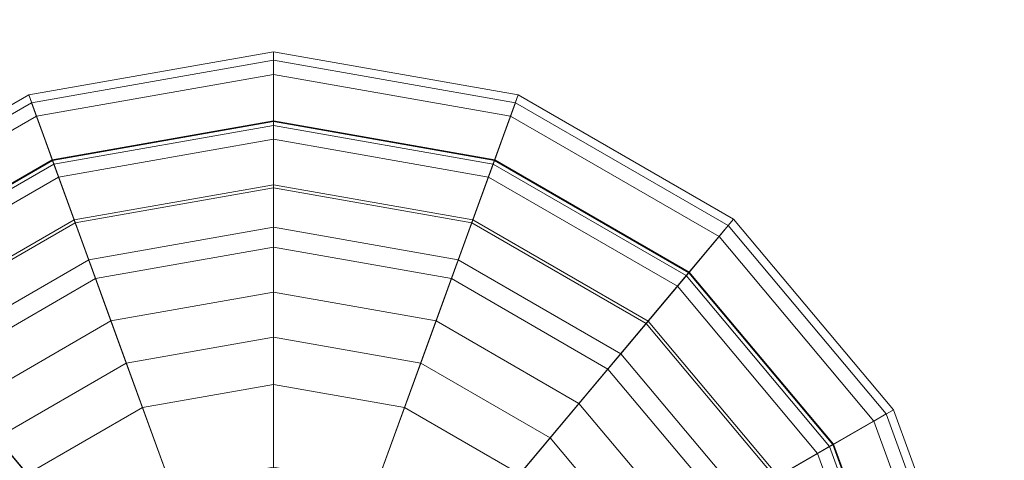
# Model space of a CAD drawing. Units: inches. Extents: x 375 to 1122, y 27 to 1069.
# Tile 131 of 155: x 721.601 to 723.463, y 903.075 to 903.908. Entities that reach past the tile are written whole.
import ezdxf

# ---------------------------------------------------------------- set-up
doc = ezdxf.new("R2010")
doc.units = ezdxf.units.IN
doc.layers.add('A-ANNO-DIMS', color=2, linetype='Continuous', lineweight=18)
doc.layers.add('Furniture', color=30, linetype='Continuous', lineweight=18)
doc.styles.get("Standard").update_dxf_attribs({"font": 'arial.ttf'})
doc.dimstyles.new('ISO-25', dxfattribs={"dimtxt": 12, "dimasz": 2.5, "dimexe": 1.5, "dimexo": 1.5, "dimtad": 1, "dimdec": 1, "dimlunit": 3, "dimtxsty": 'Standard', "dimblk": 'ARCHTICK', "dimcen": 2.5, "dimadec": 0, "dimazin": 0, "dimtfac": 1, "dimtdec": 1, "dimtmove": 0, "dimatfit": 3, "dimfxl": 1.5, "dimfxlon": 1, "dimarcsym": 0})

# ---------------------------------------------------------------- blocks, each defined once
blk = doc.blocks.new('A$C403C54AD')
at = {"linetype": 'ByBlock', "invisible_edges": 5}
for points in [[(0.818605, 0.976049, -0.033549), (0.847931, 0.959118, -0.024314), (0.86649, 1.028382, -0.024314), (0.832628, 1.028382, -0.033549)], [(0.847931, 0.959118, -0.019696), (0.831935, 0.968354, -0.019696), (0.84802, 1.028382, -0.019696), (0.86649, 1.028382, -0.019696)]]:
    blk.add_3dface(points, dxfattribs=at)
at = {"linetype": 'ByBlock'}
blk.add_3dface([(0.847931, 0.959118, -0.024314), (0.847931, 0.959118, -0.019696), (0.86649, 1.028382, -0.019696), (0.86649, 1.028382, -0.024314)], dxfattribs=at)
for points in [[(0.890422, 0.958466, -0.039553), (0.889855, 0.961682, -0.042784), (0.878804, 0.95766, -0.042784), (0.880436, 0.954832, -0.039553)], [(0.889855, 0.961682, -0.042784), (0.895735, 0.928335, -0.039705), (0.895735, 0.928335, -0.039705), (0.878804, 0.95766, -0.042784)], [(0.890429, 0.958426, 0.1202), (0.889924, 0.961289, 0.106976), (0.879003, 0.957315, 0.106976), (0.880457, 0.954797, 0.1202)], [(0.889924, 0.961289, 0.106976), (0.890041, 0.960625, 0.078734), (0.87934, 0.95673, 0.078734), (0.879003, 0.957315, 0.106976)], [(0.890041, 0.960625, 0.078734), (0.890973, 0.955342, 0.060725), (0.882023, 0.952084, 0.060725), (0.87934, 0.95673, 0.078734)], [(0.893266, 0.942333, -0.036278), (0.890422, 0.958466, -0.039553), (0.880436, 0.954832, -0.039553), (0.888627, 0.940645, -0.036278)], [(0.891296, 0.953506, 0.129606), (0.890429, 0.958426, 0.1202), (0.880457, 0.954797, 0.1202), (0.882955, 0.95047, 0.129606)], [(0.890459, 0.958252, 0.106759), (0.890947, 0.955485, 0.119395), (0.88195, 0.95221, 0.119395), (0.880545, 0.954643, 0.106759)], [(0.890574, 0.957604, 0.079219), (0.890459, 0.958252, 0.106759), (0.880545, 0.954643, 0.106759), (0.880874, 0.954073, 0.079219)], [(0.880436, 0.954832, -0.039553), (0.878804, 0.95766, -0.042784), (0.869795, 0.950101, -0.042784), (0.872296, 0.948002, -0.039553)], [(0.878804, 0.95766, -0.042784), (0.895735, 0.928335, -0.039705), (0.895735, 0.928335, -0.039705), (0.869795, 0.950101, -0.042784)], [(0.880457, 0.954797, 0.1202), (0.879003, 0.957315, 0.106976), (0.8701, 0.949844, 0.106976), (0.872327, 0.947976, 0.1202)], [(0.879003, 0.957315, 0.106976), (0.87934, 0.95673, 0.078734), (0.870617, 0.949411, 0.078734), (0.8701, 0.949844, 0.106976)], [(0.891461, 0.952574, 0.062072), (0.890574, 0.957604, 0.079219), (0.880874, 0.954073, 0.079219), (0.883428, 0.94965, 0.062072)], [(0.87934, 0.95673, 0.078734), (0.882023, 0.952084, 0.060725), (0.874727, 0.945962, 0.060725), (0.870617, 0.949411, 0.078734)], [(0.888627, 0.940645, -0.036278), (0.880436, 0.954832, -0.039553), (0.872296, 0.948002, -0.039553), (0.884846, 0.937471, -0.036278)], [(0.882955, 0.95047, 0.129606), (0.880457, 0.954797, 0.1202), (0.872327, 0.947976, 0.1202), (0.876155, 0.944764, 0.129606)], [(0.880545, 0.954643, 0.106759), (0.88195, 0.95221, 0.119395), (0.874615, 0.946056, 0.119395), (0.872463, 0.947862, 0.106759)], [(0.880874, 0.954073, 0.079219), (0.880545, 0.954643, 0.106759), (0.872463, 0.947862, 0.106759), (0.872967, 0.947439, 0.079219)], [(0.883428, 0.94965, 0.062072), (0.880874, 0.954073, 0.079219), (0.872967, 0.947439, 0.079219), (0.87688, 0.944156, 0.062072)], [(0.88195, 0.95221, 0.119395), (0.884494, 0.947804, 0.129606), (0.878513, 0.942785, 0.129606), (0.874615, 0.946056, 0.119395)], [(0.882023, 0.952084, 0.060725), (0.885556, 0.945965, 0.050493), (0.88014, 0.94142, 0.050493), (0.874727, 0.945962, 0.060725)], [(0.884494, 0.947804, 0.129606), (0.882955, 0.95047, 0.129606), (0.876155, 0.944764, 0.129606), (0.878513, 0.942785, 0.129606)], [(0.872296, 0.948002, -0.039553), (0.869795, 0.950101, -0.042784), (0.863915, 0.939916, -0.042784), (0.866983, 0.938799, -0.039553)], [(0.869795, 0.950101, -0.042784), (0.895735, 0.928335, -0.039705), (0.895735, 0.928335, -0.039705), (0.863915, 0.939916, -0.042784)], [(0.872327, 0.947976, 0.1202), (0.8701, 0.949844, 0.106976), (0.864289, 0.93978, 0.106976), (0.867021, 0.938785, 0.1202)], [(0.8701, 0.949844, 0.106976), (0.870617, 0.949411, 0.078734), (0.864924, 0.939549, 0.078734), (0.864289, 0.93978, 0.106976)], [(0.870617, 0.949411, 0.078734), (0.874727, 0.945962, 0.060725), (0.869965, 0.937714, 0.060725), (0.864924, 0.939549, 0.078734)], [(0.886671, 0.944033, 0.05268), (0.883428, 0.94965, 0.062072), (0.87688, 0.944156, 0.062072), (0.881848, 0.939987, 0.05268)], [(0.884846, 0.937471, -0.036278), (0.872296, 0.948002, -0.039553), (0.866983, 0.938799, -0.039553), (0.882378, 0.933196, -0.036278)], [(0.876155, 0.944764, 0.129606), (0.872327, 0.947976, 0.1202), (0.867021, 0.938785, 0.1202), (0.871716, 0.937076, 0.129606)], [(0.872463, 0.947862, 0.106759), (0.874615, 0.946056, 0.119395), (0.869828, 0.937764, 0.119395), (0.867188, 0.938725, 0.106759)], [(0.872967, 0.947439, 0.079219), (0.872463, 0.947862, 0.106759), (0.867188, 0.938725, 0.106759), (0.867806, 0.9385, 0.079219)], [(0.87688, 0.944156, 0.062072), (0.872967, 0.947439, 0.079219), (0.867806, 0.9385, 0.079219), (0.872606, 0.936753, 0.062072)], [(0.874615, 0.946056, 0.119395), (0.878513, 0.942785, 0.129606), (0.874609, 0.936024, 0.129606), (0.869828, 0.937764, 0.119395)], [(0.874727, 0.945962, 0.060725), (0.88014, 0.94142, 0.050493), (0.876605, 0.935297, 0.050493), (0.869965, 0.937714, 0.060725)], [(0.885556, 0.945965, 0.050493), (0.890675, 0.937098, 0.043125), (0.887983, 0.934839, 0.043125), (0.88014, 0.94142, 0.050493)], [(0.878513, 0.942785, 0.129606), (0.876155, 0.944764, 0.129606), (0.871716, 0.937076, 0.129606), (0.874609, 0.936024, 0.129606)], [(0.881848, 0.939987, 0.05268), (0.87688, 0.944156, 0.062072), (0.872606, 0.936753, 0.062072), (0.878701, 0.934534, 0.05268)], [(0.88014, 0.94142, 0.050493), (0.887983, 0.934839, 0.043125), (0.886226, 0.931795, 0.043125), (0.876605, 0.935297, 0.050493)], [(0.888914, 0.934058, 0.046044), (0.881848, 0.939987, 0.05268), (0.878701, 0.934534, 0.05268), (0.887368, 0.93138, 0.046044)], [(0.863915, 0.939916, -0.042784), (0.895735, 0.928335, -0.039705), (0.895735, 0.928335, -0.039705), (0.861872, 0.928335, -0.042784)], [(0.866983, 0.938799, -0.039553), (0.863915, 0.939916, -0.042784), (0.861872, 0.928335, -0.042784), (0.865138, 0.928335, -0.039553)], [(0.867021, 0.938785, 0.1202), (0.864289, 0.93978, 0.106976), (0.862271, 0.928335, 0.106976), (0.865179, 0.928335, 0.1202)], [(0.864289, 0.93978, 0.106976), (0.864924, 0.939549, 0.078734), (0.862946, 0.928335, 0.078734), (0.862271, 0.928335, 0.106976)], [(0.864924, 0.939549, 0.078734), (0.869965, 0.937714, 0.060725), (0.868311, 0.928335, 0.060725), (0.862946, 0.928335, 0.078734)], [(0.882378, 0.933196, -0.036278), (0.866983, 0.938799, -0.039553), (0.865138, 0.928335, -0.039553), (0.88152, 0.928335, -0.036278)], [(0.871716, 0.937076, 0.129606), (0.867021, 0.938785, 0.1202), (0.865179, 0.928335, 0.1202), (0.870175, 0.928335, 0.129606)], [(0.867188, 0.938725, 0.106759), (0.869828, 0.937764, 0.119395), (0.868166, 0.928335, 0.119395), (0.865356, 0.928335, 0.106759)], [(0.867806, 0.9385, 0.079219), (0.867188, 0.938725, 0.106759), (0.865356, 0.928335, 0.106759), (0.866014, 0.928335, 0.079219)], [(0.872606, 0.936753, 0.062072), (0.867806, 0.9385, 0.079219), (0.866014, 0.928335, 0.079219), (0.871122, 0.928335, 0.062072)], [(0.869828, 0.937764, 0.119395), (0.874609, 0.936024, 0.129606), (0.873253, 0.928335, 0.129606), (0.868166, 0.928335, 0.119395)], [(0.869965, 0.937714, 0.060725), (0.876605, 0.935297, 0.050493), (0.875377, 0.928335, 0.050493), (0.868311, 0.928335, 0.060725)], [(0.874609, 0.936024, 0.129606), (0.871716, 0.937076, 0.129606), (0.870175, 0.928335, 0.129606), (0.873253, 0.928335, 0.129606)], [(0.878701, 0.934534, 0.05268), (0.872606, 0.936753, 0.062072), (0.871122, 0.928335, 0.062072), (0.877607, 0.928335, 0.05268)], [(0.876605, 0.935297, 0.050493), (0.886226, 0.931795, 0.043125), (0.885616, 0.928335, 0.043125), (0.875377, 0.928335, 0.050493)], [(0.887368, 0.93138, 0.046044), (0.878701, 0.934534, 0.05268), (0.877607, 0.928335, 0.05268), (0.886831, 0.928335, 0.046044)], [(0.861872, 0.928335, -0.042784), (0.895735, 0.928335, -0.039705), (0.895735, 0.928335, -0.039705), (0.863915, 0.916753, -0.042784)], [(0.865138, 0.928335, -0.039553), (0.861872, 0.928335, -0.042784), (0.863915, 0.916753, -0.042784), (0.866983, 0.91787, -0.039553)], [(0.865179, 0.928335, 0.1202), (0.862271, 0.928335, 0.106976), (0.864289, 0.916889, 0.106976), (0.867021, 0.917884, 0.1202)], [(0.862271, 0.928335, 0.106976), (0.862946, 0.928335, 0.078734), (0.864924, 0.91712, 0.078734), (0.864289, 0.916889, 0.106976)], [(0.862946, 0.928335, 0.078734), (0.868311, 0.928335, 0.060725), (0.869965, 0.918955, 0.060725), (0.864924, 0.91712, 0.078734)], [(0.863915, 0.916753, -0.042784), (0.895735, 0.928335, -0.039705), (0.895735, 0.928335, -0.039705), (0.869795, 0.906568, -0.042784)], [(0.88152, 0.928335, -0.036278), (0.865138, 0.928335, -0.039553), (0.866983, 0.91787, -0.039553), (0.882378, 0.923473, -0.036278)], [(0.870175, 0.928335, 0.129606), (0.865179, 0.928335, 0.1202), (0.867021, 0.917884, 0.1202), (0.871716, 0.919593, 0.129606)], [(0.865356, 0.928335, 0.106759), (0.868166, 0.928335, 0.119395), (0.869828, 0.918905, 0.119395), (0.867188, 0.917944, 0.106759)], [(0.866014, 0.928335, 0.079219), (0.865356, 0.928335, 0.106759), (0.867188, 0.917944, 0.106759), (0.867806, 0.918169, 0.079219)], [(0.871122, 0.928335, 0.062072), (0.866014, 0.928335, 0.079219), (0.867806, 0.918169, 0.079219), (0.872606, 0.919916, 0.062072)], [(0.868166, 0.928335, 0.119395), (0.873253, 0.928335, 0.129606), (0.874609, 0.920646, 0.129606), (0.869828, 0.918905, 0.119395)], [(0.868311, 0.928335, 0.060725), (0.875377, 0.928335, 0.050493), (0.876605, 0.921372, 0.050493), (0.869965, 0.918955, 0.060725)], [(0.869795, 0.906568, -0.042784), (0.895735, 0.928335, -0.039705), (0.895735, 0.928335, -0.039705), (0.878804, 0.899009, -0.042784)], [(0.873253, 0.928335, 0.129606), (0.870175, 0.928335, 0.129606), (0.871716, 0.919593, 0.129606), (0.874609, 0.920646, 0.129606)], [(0.877607, 0.928335, 0.05268), (0.871122, 0.928335, 0.062072), (0.872606, 0.919916, 0.062072), (0.878701, 0.922135, 0.05268)], [(0.875377, 0.928335, 0.050493), (0.885616, 0.928335, 0.043125), (0.886226, 0.924874, 0.043125), (0.876605, 0.921372, 0.050493)], [(0.886831, 0.928335, 0.046044), (0.877607, 0.928335, 0.05268), (0.878701, 0.922135, 0.05268), (0.887368, 0.925289, 0.046044)], [(0.878804, 0.899009, -0.042784), (0.895735, 0.928335, -0.039705), (0.895735, 0.928335, -0.039705), (0.889855, 0.894987, -0.042784)], [(0.887368, 0.925289, 0.046044), (0.878701, 0.922135, 0.05268), (0.881848, 0.916683, 0.05268), (0.888914, 0.922611, 0.046044)], [(0.876605, 0.921372, 0.050493), (0.886226, 0.924874, 0.043125), (0.887983, 0.92183, 0.043125), (0.88014, 0.915249, 0.050493)], [(0.882378, 0.923473, -0.036278), (0.866983, 0.91787, -0.039553), (0.872296, 0.908668, -0.039553), (0.884846, 0.919198, -0.036278)], [(0.878701, 0.922135, 0.05268), (0.872606, 0.919916, 0.062072), (0.87688, 0.912514, 0.062072), (0.881848, 0.916683, 0.05268)], [(0.88014, 0.915249, 0.050493), (0.887983, 0.92183, 0.043125), (0.890675, 0.919571, 0.043125), (0.885556, 0.910704, 0.050493)], [(0.869965, 0.918955, 0.060725), (0.876605, 0.921372, 0.050493), (0.88014, 0.915249, 0.050493), (0.874727, 0.910707, 0.060725)], [(0.869828, 0.918905, 0.119395), (0.874609, 0.920646, 0.129606), (0.878513, 0.913884, 0.129606), (0.874615, 0.910614, 0.119395)], [(0.874609, 0.920646, 0.129606), (0.871716, 0.919593, 0.129606), (0.876155, 0.911905, 0.129606), (0.878513, 0.913884, 0.129606)], [(0.872606, 0.919916, 0.062072), (0.867806, 0.918169, 0.079219), (0.872967, 0.90923, 0.079219), (0.87688, 0.912514, 0.062072)], [(0.871716, 0.919593, 0.129606), (0.867021, 0.917884, 0.1202), (0.872327, 0.908694, 0.1202), (0.876155, 0.911905, 0.129606)], [(0.884846, 0.919198, -0.036278), (0.872296, 0.908668, -0.039553), (0.880436, 0.901837, -0.039553), (0.888627, 0.916025, -0.036278)], [(0.864924, 0.91712, 0.078734), (0.869965, 0.918955, 0.060725), (0.874727, 0.910707, 0.060725), (0.870617, 0.907259, 0.078734)], [(0.867188, 0.917944, 0.106759), (0.869828, 0.918905, 0.119395), (0.874615, 0.910614, 0.119395), (0.872463, 0.908807, 0.106759)], [(0.867806, 0.918169, 0.079219), (0.867188, 0.917944, 0.106759), (0.872463, 0.908807, 0.106759), (0.872967, 0.90923, 0.079219)], [(0.866983, 0.91787, -0.039553), (0.863915, 0.916753, -0.042784), (0.869795, 0.906568, -0.042784), (0.872296, 0.908668, -0.039553)], [(0.867021, 0.917884, 0.1202), (0.864289, 0.916889, 0.106976), (0.8701, 0.906825, 0.106976), (0.872327, 0.908694, 0.1202)], [(0.864289, 0.916889, 0.106976), (0.864924, 0.91712, 0.078734), (0.870617, 0.907259, 0.078734), (0.8701, 0.906825, 0.106976)], [(0.881848, 0.916683, 0.05268), (0.87688, 0.912514, 0.062072), (0.883428, 0.907019, 0.062072), (0.886671, 0.912636, 0.05268)]]:
    blk.add_3dface(points)
blk = doc.blocks.new('_ArchTick')
at = {"color": 0, "linetype": 'ByBlock', "const_width": 0.15}
blk.add_lwpolyline([(-0.5, -0.5), (0.5, 0.5)], dxfattribs=at)
blk = doc.blocks.new('*D73')
at = {"layer": 'A-ANNO-DIMS', "color": 0, "lineweight": -2, "transparency": 16777216}
for p, q in [((686.7573, 932.4277), (686.7573, 929.4277)), ((770.7573, 932.4277), (770.7573, 929.4277)), ((686.7573, 930.9277), (770.7573, 930.9277)), ((770.7573, 930.9277), (987.6096, 930.9277))]:
    blk.add_line(p, q, dxfattribs=at)
at = {"layer": 'Defpoints', "color": 0, "transparency": 16777216}
for p in [(686.7573, 943.5277), (770.7573, 943.5277), (770.7573, 930.9277)]:
    blk.add_point(p, dxfattribs=at)
at = {"layer": 'A-ANNO-DIMS', "color": 0, "lineweight": -2, "transparency": 16777216, "xscale": 2.5, "yscale": 2.5, "zscale": 2.5, "rotation": 180}
blk.add_blockref('_ArchTick', (686.7573, 930.9277), dxfattribs=at)
at = {"layer": 'A-ANNO-DIMS', "color": 0, "lineweight": -2, "transparency": 16777216, "xscale": 2.5, "yscale": 2.5, "zscale": 2.5}
blk.add_blockref('_ArchTick', (770.7573, 930.9277), dxfattribs=at)
at = {"layer": 'A-ANNO-DIMS', "color": 0, "transparency": 16777216, "insert": (880.4335, 937.7573), "char_height": 12, "attachment_point": 5}
blk.add_mtext('2-PANEL SLIDER 7\'-0" TYP.', dxfattribs=at)

msp = doc.modelspace()

# ---------------------------------------------------------------- block references
at = {"layer": 'Furniture', "xscale": 39.9918517141215, "yscale": 39.9918517141215, "zscale": 39.9918517141215, "rotation": 270}
msp.add_blockref('A$C403C54AD', (684.9549, 938.3156, 0.024), dxfattribs=at)

# ---------------------------------------------------------------- dimensions: what is measured, and where the dimension line sits
at = {"layer": 'A-ANNO-DIMS'}
dim = msp.add_linear_dim(base=(770.7573, 930.9277), p1=(686.7573, 943.5277), p2=(770.7573, 943.5277), text='2-PANEL SLIDER <> TYP.', dimstyle='ISO-25', override={"dimdec": 1, "dimlfac": 1, "dimrnd": 0, "dimzin": 1, "dimdsep": 46, "dimlunit": 4, "dimfrac": 2}, dxfattribs=at)
dim.commit()
dim.dimension.update_dxf_attribs({"geometry": '*D73', "text_midpoint": (880.4335, 937.7573)})

doc.saveas('drawing.dxf')
